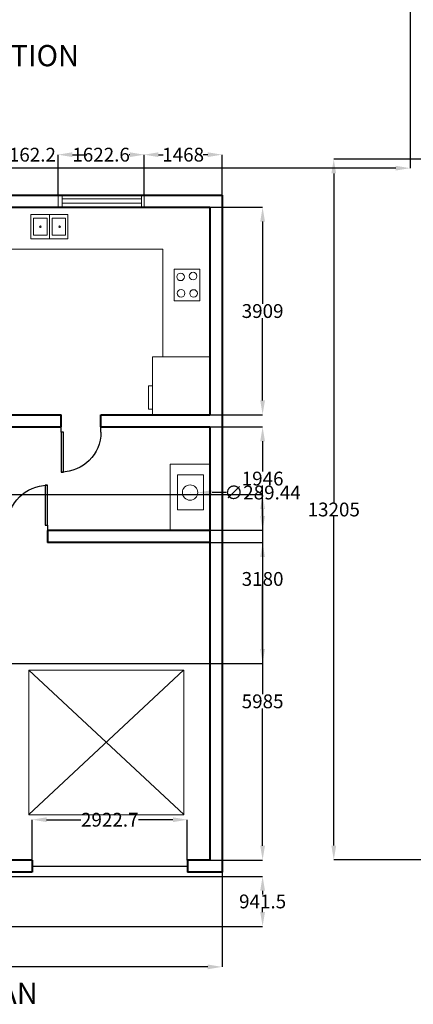
# Model space of a CAD drawing. Units: millimetres. Extents: x 23 to 3809233, y 4 to 290343.
# Tile 3 of 8: x 1908235 to 1915648, y 133276 to 151826. Entities that reach past the tile are written whole.
import ezdxf

# ---------------------------------------------------------------- set-up
doc = ezdxf.new("R2010")
doc.units = ezdxf.units.MM
doc.header["$MEASUREMENT"] = 0
for name, color, linetype, lineweight in [('A-ANNO-DIMS', 2, 'Continuous', 18), ('A-ANNO-TEXT', 7, 'Continuous', 25), ('A-DOOR', 3, 'Continuous', 25), ('A-EQPM', 8, 'Continuous', 18), ('A-FLOR-CASE', 8, 'Continuous', 20), ('A-FLOR-FIXT', 9, 'Continuous', 18), ('A-GLAZ', 4, 'Continuous', 18), ('A-WALL', 7, 'Continuous', 40)]:
    doc.layers.add(name, color=color, linetype=linetype, lineweight=lineweight)
doc.styles.get("Standard").update_dxf_attribs({"font": 'arial.ttf'})
doc.dimstyles.get("Standard").update_dxf_attribs({"dimtxt": 260.18, "dimasz": 270.18, "dimexe": 0.18, "dimexo": 0.0625, "dimgap": 0.09, "dimtad": 0, "dimtih": 1, "dimtoh": 1, "dimdec": 0, "dimzin": 0, "dimdsep": 46, "dimtxsty": 'Standard', "dimcen": 0.09, "dimadec": 0, "dimazin": 0, "dimtfac": 1, "dimtdec": 0, "dimtofl": 0, "dimtmove": 0, "dimatfit": 3, "dimfxl": 1, "dimtolj": 1, "dimtzin": 0, "dimarcsym": 0})

# ---------------------------------------------------------------- blocks, each defined once
blk = doc.blocks.new('*U2')
for p, q in [((0, 0), (0, -100)), ((750, 0), (750, -100))]:
    blk.add_line(p, q)
blk.add_lwpolyline([(0, 0), (0, 750), (43.75, 750), (43.75, 0)], close=True)
blk.add_arc((0, 0), 750, 0, 90)
blk = doc.blocks.new('*D48')
at = {"layer": 'A-ANNO-DIMS', "color": 0, "lineweight": -2, "transparency": 16777216}
for p, q in [((1898390, 135763), (1898390, 133980)), ((1912047, 135763), (1912047, 133980)), ((1898660, 133981), (1904741, 133981)), ((1911777, 133981), (1905696, 133981))]:
    blk.add_line(p, q, dxfattribs=at)
at = {"layer": 'A-ANNO-DIMS', "color": 0, "transparency": 16777216}
for points in [[(1898660, 134026), (1898660, 133936), (1898390, 133981)], [(1911777, 134026), (1911777, 133936), (1912047, 133981)]]:
    blk.add_solid(points, dxfattribs=at)
at = {"layer": 'Defpoints', "color": 0, "transparency": 16777216}
for p in [(1898390, 135763), (1912047, 135763), (1912047, 133981)]:
    blk.add_point(p, dxfattribs=at)
at = {"layer": 'A-ANNO-DIMS', "color": 0, "transparency": 16777216, "insert": (1905219, 133981), "char_height": 260.2, "attachment_point": 5}
blk.add_mtext('\\A1;13657', dxfattribs=at)
blk = doc.blocks.new('*D53')
at = {"layer": 'A-ANNO-DIMS', "color": 0, "lineweight": -2, "transparency": 16777216}
for p, q in [((1911819, 141976), (1912810, 141976)), ((1912810, 141706), (1912810, 139117)), ((1912810, 136262), (1912810, 138851)), ((1911819, 135992), (1912810, 135992))]:
    blk.add_line(p, q, dxfattribs=at)
at = {"layer": 'A-ANNO-DIMS', "color": 0, "transparency": 16777216}
for points in [[(1912765, 141706), (1912855, 141706), (1912810, 141976)], [(1912765, 136262), (1912855, 136262), (1912810, 135992)]]:
    blk.add_solid(points, dxfattribs=at)
at = {"layer": 'Defpoints', "color": 0, "transparency": 16777216}
for p in [(1911819, 141976), (1912810, 141976), (1911819, 135992)]:
    blk.add_point(p, dxfattribs=at)
at = {"layer": 'A-ANNO-DIMS', "color": 0, "transparency": 16777216, "insert": (1912810, 138984), "char_height": 260.2, "attachment_point": 5}
blk.add_mtext('\\A1;5985', dxfattribs=at)
blk = doc.blocks.new('*D54')
at = {"layer": 'A-ANNO-DIMS', "color": 0, "lineweight": -2, "transparency": 16777216}
for p, q in [((1911819, 144154), (1912810, 144154)), ((1912810, 143884), (1912810, 143314)), ((1912810, 142478), (1912810, 143048)), ((1911816, 142208), (1912810, 142208))]:
    blk.add_line(p, q, dxfattribs=at)
at = {"layer": 'A-ANNO-DIMS', "color": 0, "transparency": 16777216}
for points in [[(1912765, 143884), (1912855, 143884), (1912810, 144154)], [(1912765, 142478), (1912855, 142478), (1912810, 142208)]]:
    blk.add_solid(points, dxfattribs=at)
at = {"layer": 'Defpoints', "color": 0, "transparency": 16777216}
for p in [(1911819, 144154), (1912810, 144154), (1911816, 142208)]:
    blk.add_point(p, dxfattribs=at)
at = {"layer": 'A-ANNO-DIMS', "color": 0, "transparency": 16777216, "insert": (1912810, 143181), "char_height": 260.2, "attachment_point": 5}
blk.add_mtext('\\A1;1946', dxfattribs=at)
blk = doc.blocks.new('*D55')
at = {"layer": 'A-ANNO-DIMS', "color": 0, "lineweight": -2, "transparency": 16777216}
for p, q in [((1911819, 148292), (1912810, 148292)), ((1912810, 148022), (1912810, 146470)), ((1912810, 144653), (1912810, 146204)), ((1911816, 144382), (1912810, 144382))]:
    blk.add_line(p, q, dxfattribs=at)
at = {"layer": 'A-ANNO-DIMS', "color": 0, "transparency": 16777216}
for points in [[(1912765, 148022), (1912855, 148022), (1912810, 148292)], [(1912765, 144653), (1912855, 144653), (1912810, 144382)]]:
    blk.add_solid(points, dxfattribs=at)
at = {"layer": 'Defpoints', "color": 0, "transparency": 16777216}
for p in [(1911819, 148292), (1912810, 148292), (1911816, 144382)]:
    blk.add_point(p, dxfattribs=at)
at = {"layer": 'A-ANNO-DIMS', "color": 0, "transparency": 16777216, "insert": (1912810, 146337), "char_height": 260.2, "attachment_point": 5}
blk.add_mtext('\\A1;3909', dxfattribs=at)
blk = doc.blocks.new('*D64')
at = {"layer": 'A-ANNO-DIMS', "color": 0, "lineweight": -2, "transparency": 16777216}
for p, q in [((1907524.135363, 149282.788959), (1907253.955363, 149282.788959)), ((1907794.315363, 148291.751459), (1907794.315363, 149282.968959)), ((1908956.509231, 148520.351459), (1908956.509231, 149282.968959)), ((1909226.689231, 149282.788959), (1909496.869231, 149282.788959))]:
    blk.add_line(p, q, dxfattribs=at)
at = {"layer": 'A-ANNO-DIMS', "color": 0, "transparency": 16777216}
for points in [[(1907524.135363, 149327.818959), (1907524.135363, 149237.758959), (1907794.315363, 149282.788959)], [(1909226.689231, 149327.818959), (1909226.689231, 149237.758959), (1908956.509231, 149282.788959)]]:
    blk.add_solid(points, dxfattribs=at)
at = {"layer": 'Defpoints', "color": 0, "transparency": 16777216}
for p in [(1908956.509231, 149282.788959), (1908956.509231, 148520.288959), (1907794.315363, 148291.688959)]:
    blk.add_point(p, dxfattribs=at)
at = {"layer": 'A-ANNO-DIMS', "color": 0, "transparency": 16777216, "insert": (1908375.412297, 149282.788959), "char_height": 260.18, "attachment_point": 5}
blk.add_mtext('\\A1;1162.2', dxfattribs=at)
blk = doc.blocks.new('*D65')
at = {"layer": 'A-ANNO-DIMS', "color": 0, "lineweight": -2, "transparency": 16777216}
for p, q in [((1908957, 148520), (1908957, 149283)), ((1909227, 149283), (1909240, 149283)), ((1910309, 149283), (1910296, 149283)), ((1910579, 148520), (1910579, 149283))]:
    blk.add_line(p, q, dxfattribs=at)
at = {"layer": 'A-ANNO-DIMS', "color": 0, "transparency": 16777216}
for points in [[(1909227, 149328), (1909227, 149238), (1908957, 149283)], [(1910309, 149328), (1910309, 149238), (1910579, 149283)]]:
    blk.add_solid(points, dxfattribs=at)
at = {"layer": 'Defpoints', "color": 0, "transparency": 16777216}
for p in [(1910579, 149283), (1908957, 148520), (1910579, 148520)]:
    blk.add_point(p, dxfattribs=at)
at = {"layer": 'A-ANNO-DIMS', "color": 0, "transparency": 16777216, "insert": (1909768, 149283), "char_height": 260.2, "attachment_point": 5}
blk.add_mtext('\\A1;1622.6', dxfattribs=at)
blk = doc.blocks.new('*D66')
at = {"layer": 'A-ANNO-DIMS', "color": 0, "lineweight": -2, "transparency": 16777216}
for p, q in [((1910579, 148520), (1910579, 149283)), ((1910849, 149283), (1910937, 149283)), ((1911777, 149283), (1911690, 149283)), ((1912047, 148520), (1912047, 149283))]:
    blk.add_line(p, q, dxfattribs=at)
at = {"layer": 'A-ANNO-DIMS', "color": 0, "transparency": 16777216}
for points in [[(1910849, 149328), (1910849, 149238), (1910579, 149283)], [(1911777, 149328), (1911777, 149238), (1912047, 149283)]]:
    blk.add_solid(points, dxfattribs=at)
at = {"layer": 'Defpoints', "color": 0, "transparency": 16777216}
for p in [(1912047, 149283), (1910579, 148520), (1912047, 148520)]:
    blk.add_point(p, dxfattribs=at)
at = {"layer": 'A-ANNO-DIMS', "color": 0, "transparency": 16777216, "insert": (1911313, 149283), "char_height": 260.2, "attachment_point": 5}
blk.add_mtext('\\A1;1468', dxfattribs=at)
blk = doc.blocks.new('*D69')
at = {"layer": 'A-ANNO-DIMS', "color": 0, "lineweight": -2, "transparency": 16777216}
for p, q in [((1908470, 135992), (1908470, 136754)), ((1908740, 136754), (1909389, 136754)), ((1911122, 136754), (1910473, 136754)), ((1911392, 135992), (1911392, 136754))]:
    blk.add_line(p, q, dxfattribs=at)
at = {"layer": 'A-ANNO-DIMS', "color": 0, "transparency": 16777216}
for points in [[(1908740, 136799), (1908740, 136709), (1908470, 136754)], [(1911122, 136799), (1911122, 136709), (1911392, 136754)]]:
    blk.add_solid(points, dxfattribs=at)
at = {"layer": 'Defpoints', "color": 0, "transparency": 16777216}
for p in [(1911392, 136754), (1908470, 135992), (1911392, 135992)]:
    blk.add_point(p, dxfattribs=at)
at = {"layer": 'A-ANNO-DIMS', "color": 0, "transparency": 16777216, "insert": (1909931, 136754), "char_height": 260.2, "attachment_point": 5}
blk.add_mtext('\\A1;2922.7', dxfattribs=at)
blk = doc.blocks.new('*D71')
at = {"layer": 'A-ANNO-DIMS', "color": 0, "lineweight": -2, "transparency": 16777216}
for p, q in [((1905183, 142880), (1912810, 142880)), ((1912810, 142610), (1912810, 141423)), ((1912810, 139970), (1912810, 141157)), ((1905183, 139700), (1912810, 139700))]:
    blk.add_line(p, q, dxfattribs=at)
at = {"layer": 'A-ANNO-DIMS', "color": 0, "transparency": 16777216}
for points in [[(1912765, 142610), (1912855, 142610), (1912810, 142880)], [(1912765, 139970), (1912855, 139970), (1912810, 139700)]]:
    blk.add_solid(points, dxfattribs=at)
at = {"layer": 'Defpoints', "color": 0, "transparency": 16777216}
for p in [(1905183, 142880), (1912810, 142880), (1905183, 139700)]:
    blk.add_point(p, dxfattribs=at)
at = {"layer": 'A-ANNO-DIMS', "color": 0, "transparency": 16777216, "insert": (1912810, 141290), "char_height": 260.2, "attachment_point": 5}
blk.add_mtext('\\A1;3180', dxfattribs=at)
blk = doc.blocks.new('*D79')
at = {"layer": 'A-ANNO-DIMS', "color": 0, "lineweight": -2, "transparency": 16777216}
for p, q in [((1906678, 135685), (1912810, 135685)), ((1912810, 135414), (1912810, 135347)), ((1912810, 135013), (1912810, 135081)), ((1906678, 134743), (1912810, 134743))]:
    blk.add_line(p, q, dxfattribs=at)
at = {"layer": 'A-ANNO-DIMS', "color": 0, "transparency": 16777216}
for points in [[(1912765, 135414), (1912855, 135414), (1912810, 135685)], [(1912765, 135013), (1912855, 135013), (1912810, 134743)]]:
    blk.add_solid(points, dxfattribs=at)
at = {"layer": 'Defpoints', "color": 0, "transparency": 16777216}
for p in [(1906678, 135685), (1912810, 135685), (1906678, 134743)]:
    blk.add_point(p, dxfattribs=at)
at = {"layer": 'A-ANNO-DIMS', "color": 0, "transparency": 16777216, "insert": (1912810, 135214), "char_height": 260.2, "attachment_point": 5}
blk.add_mtext('\\A1;941.5', dxfattribs=at)
blk = doc.blocks.new('*D80')
at = {"layer": 'A-ANNO-DIMS', "color": 0, "lineweight": -2, "transparency": 16777216}
for p, q in [((1893468, 163690), (1893468, 149029)), ((1915588, 152264), (1915588, 149029)), ((1893739, 149029), (1904037, 149029)), ((1915318, 149029), (1905020, 149029))]:
    blk.add_line(p, q, dxfattribs=at)
at = {"layer": 'A-ANNO-DIMS', "color": 0, "transparency": 16777216}
for points in [[(1893739, 149074), (1893739, 148984), (1893468, 149029)], [(1915318, 149074), (1915318, 148984), (1915588, 149029)]]:
    blk.add_solid(points, dxfattribs=at)
at = {"layer": 'Defpoints', "color": 0, "transparency": 16777216}
for p in [(1893468, 163690), (1915588, 152265), (1915588, 149029)]:
    blk.add_point(p, dxfattribs=at)
at = {"layer": 'A-ANNO-DIMS', "color": 0, "transparency": 16777216, "insert": (1904528, 149029), "char_height": 260.2, "attachment_point": 5}
blk.add_mtext('\\A1;22120', dxfattribs=at)
blk = doc.blocks.new('*D117')
at = {"layer": 'A-ANNO-DIMS', "color": 0, "lineweight": -2, "transparency": 16777216}
for p, q in [((1929762, 149200), (1914150, 149200)), ((1914150, 148930), (1914150, 142731)), ((1914150, 136265), (1914150, 142465)), ((1918411, 135995), (1914150, 135995))]:
    blk.add_line(p, q, dxfattribs=at)
at = {"layer": 'A-ANNO-DIMS', "color": 0, "transparency": 16777216}
for points in [[(1914105, 148930), (1914195, 148930), (1914150, 149200)], [(1914105, 136265), (1914195, 136265), (1914150, 135995)]]:
    blk.add_solid(points, dxfattribs=at)
at = {"layer": 'Defpoints', "color": 0, "transparency": 16777216}
for p in [(1914150, 149200), (1929762, 149200), (1918411, 135995)]:
    blk.add_point(p, dxfattribs=at)
at = {"layer": 'A-ANNO-DIMS', "color": 0, "transparency": 16777216, "insert": (1914150, 142598), "char_height": 260.2, "attachment_point": 5}
blk.add_mtext('\\A1;13205', dxfattribs=at)
blk = doc.blocks.new('*D127')
at = {"layer": 'A-ANNO-DIMS', "color": 0, "lineweight": -2, "transparency": 16777216}
for p, q in [((1911443, 142918), (1911443, 142918)), ((1911443, 142918), (1911443, 142918)), ((1912128, 142918), (1911858, 142918))]:
    blk.add_line(p, q, dxfattribs=at)
at = {"layer": 'A-ANNO-DIMS', "color": 0, "transparency": 16777216}
blk.add_solid([(1911858, 142963), (1911858, 142873), (1911588, 142918)], dxfattribs=at)
at = {"layer": 'Defpoints', "color": 0, "transparency": 16777216}
for p in [(1911298, 142918), (1911588, 142918)]:
    blk.add_point(p, dxfattribs=at)
at = {"layer": 'A-ANNO-DIMS', "color": 0, "transparency": 16777216, "insert": (1912809, 142918), "char_height": 260.18, "attachment_point": 5}
blk.add_mtext('\\A1;∅289.44', dxfattribs=at)

msp = doc.modelspace()

# ---------------------------------------------------------------- linework, layer by layer
at = {"layer": 'A-DOOR'}
msp.add_line((1908469.731, 135877.389), (1911392.434, 135877.389), dxfattribs=at)
at = {"layer": 'A-EQPM'}
for p, q in [((1908409.259, 139573.019), (1911323.873, 136849.314)), ((1911320.873, 139573.019), (1908409.259, 136849.314))]:
    msp.add_line(p, q, dxfattribs=at)
for points in [[(1911143.931, 147120.08, -0.414213562), (1911146.931, 147123.08), (1911626.738, 147123.08, -0.414213562), (1911629.738, 147120.08), (1911629.738, 146530.897, -0.414213562), (1911626.738, 146527.897), (1911146.931, 146527.897, -0.414213562), (1911143.931, 146530.897)], [(1911818.654, 145472.116, 0.414213562), (1911815.654, 145475.116), (1910736.868, 145475.116, 0.414213562), (1910733.868, 145472.116), (1910733.868, 144385.478, 0.414213562), (1910736.868, 144382.478), (1911815.654, 144382.478, 0.414213562), (1911818.654, 144385.478)], [(1910733.868, 144925.797, 0.414213562), (1910730.868, 144928.797), (1910661.427, 144928.797, 0.414213562), (1910658.427, 144925.797), (1910658.427, 144492.893, 0.414213562), (1910661.427, 144489.893), (1910730.868, 144489.893, 0.414213562), (1910733.868, 144492.893)], [(1908406.259, 139570.019, -0.414213562), (1908409.259, 139573.019), (1911320.873, 139573.019, -0.414213562), (1911323.873, 139570.019), (1911323.873, 136849.314, -0.414213562), (1911320.873, 136846.314), (1908409.259, 136846.314, -0.414213562), (1908406.259, 136849.314)]]:
    msp.add_lwpolyline(points, format="xyb", close=True, dxfattribs=at)
for centre in [(1911265.852, 146981.031), (1911500.112, 146996.291), (1911273.49, 146670.764), (1911510.299, 146668.221)]:
    msp.add_circle(centre, 71.208, dxfattribs=at)
at = {"layer": 'A-FLOR-CASE'}
for p, q in [((1908018.892, 147503.249), (1910929.729, 147503.249)), ((1910929.729, 147503.249), (1910929.729, 145475.116)), ((1910929.729, 145475.116), (1911818.654, 145475.116))]:
    msp.add_line(p, q, dxfattribs=at)
at = {"layer": 'A-FLOR-FIXT'}
msp.add_line((1908793.459, 148156.716), (1908793.459, 147695.201), dxfattribs=at)
msp.add_lwpolyline([(1908443.683, 148156.716), (1909143.234, 148156.716), (1909143.234, 147695.201), (1908443.683, 147695.201)], close=True, dxfattribs=at)
for points in [[(1908495.983, 148083.153, -0.414213562), (1908498.983, 148086.153), (1908747.8, 148086.153, -0.414213562), (1908750.8, 148083.153), (1908750.8, 147766.619, -0.414213562), (1908747.8, 147763.619), (1908498.983, 147763.619, -0.414213562), (1908495.983, 147766.619)], [(1908843.67, 148083.153, -0.414213562), (1908846.67, 148086.153), (1909095.487, 148086.153, -0.414213562), (1909098.487, 148083.153), (1909098.487, 147766.619, -0.414213562), (1909095.487, 147763.619), (1908846.67, 147763.619, -0.414213562), (1908843.67, 147766.619)], [(1911818.654, 143448.998, 0.414213562), (1911815.654, 143451.998), (1911070.621, 143451.998, 0.414213562), (1911067.621, 143448.998), (1911067.621, 142207.876, 0.414213562), (1911070.621, 142204.876), (1911815.654, 142204.876, 0.414213562), (1911818.654, 142207.876)], [(1911694.266, 143247.447, 0.414213562), (1911691.266, 143250.447), (1911208.696, 143250.447, 0.414213562), (1911205.696, 143247.447), (1911205.696, 142595.754, 0.414213562), (1911208.696, 142592.754), (1911691.266, 142592.754, 0.414213562), (1911694.266, 142595.754)]]:
    msp.add_lwpolyline(points, format="xyb", close=True, dxfattribs=at)
for centre, radius in [((1908623.392, 147924.886), 15.119), ((1908986.197, 147924.886), 15.119), ((1911443.137, 142917.649), 144.721)]:
    msp.add_circle(centre, radius, dxfattribs=at)
at = {"layer": 'A-GLAZ'}
for p, q in [((1908956.509, 148520.289), (1908956.509, 148291.689)), ((1909037.053, 148520.289), (1909037.053, 148291.689)), ((1909037.053, 148450.918), (1910529.216, 148450.918)), ((1910529.216, 148520.289), (1910529.216, 148291.689)), ((1910579.153, 148520.289), (1910579.153, 148291.689)), ((1909037.053, 148368.638), (1910529.216, 148368.638))]:
    msp.add_line(p, q, dxfattribs=at)
at = {"layer": 'A-WALL'}
for p, q in [((1898390.054, 148520.289), (1912047.254, 148520.289)), ((1912047.254, 148520.289), (1912047.254, 135763.089)), ((1907794.315, 148291.689), (1911818.654, 148291.689)), ((1911818.654, 148291.689), (1911818.654, 144382.478)), ((1907794.315, 144382.478), (1909015.346, 144382.478)), ((1909015.346, 144153.878), (1909015.346, 144382.478)), ((1909765.346, 144153.878), (1909765.346, 144382.478)), ((1909765.346, 144382.478), (1910051.569, 144382.478)), ((1910051.569, 144382.478), (1911818.654, 144382.478)), ((1907794.315, 144153.878), (1909015.346, 144153.878)), ((1909765.346, 144153.878), (1910046.69, 144153.878)), ((1910046.69, 144153.878), (1911818.654, 144153.878)), ((1911818.654, 144153.878), (1911818.654, 135991.689)), ((1911818.654, 142577.621), (1911818.654, 135991.689)), ((1911818.654, 142204.876), (1908759.428, 142204.876)), ((1908759.428, 142204.876), (1908759.428, 141976.276)), ((1911818.654, 141976.276), (1908759.428, 141976.276)), ((1908469.731, 135991.689), (1907794.315, 135991.689)), ((1908469.731, 135991.689), (1908469.731, 135763.089)), ((1911818.654, 135991.689), (1911392.434, 135991.689)), ((1911392.434, 135991.689), (1911392.434, 135763.089)), ((1908469.731, 135763.089), (1907565.715, 135763.089)), ((1912047.254, 135763.089), (1911392.434, 135763.089))]:
    msp.add_line(p, q, dxfattribs=at)

# ---------------------------------------------------------------- block references
at = {"layer": 'A-DOOR', "xscale": -1, "rotation": 180}
msp.add_blockref('*U2', (1909015.346, 144053.878), dxfattribs=at)
at = {"layer": 'A-DOOR', "xscale": -1}
msp.add_blockref('*U2', (1908759.428, 142304.876), dxfattribs=at)

# ---------------------------------------------------------------- texts
at = {"layer": 'A-ANNO-TEXT', "char_height": 400, "attachment_point": 1}
for s, heights, insert in [('LEFT SIDE ELEVATION', [307.465], (1903808.34, 151348.696)), ('GROUND FLOOR PLAN', [0], (1902916.406, 133683.241))]:
    msp.add_mtext_dynamic_manual_height_columns(s, width=8410.77875, gutter_width=1, heights=heights, dxfattribs=dict(at, insert=insert))

# ---------------------------------------------------------------- dimensions: what is measured, and where the dimension line sits
at = {"layer": 'A-ANNO-DIMS'}
for base, p1, p2, override, picture, middle in [((1915588.32, 149029.101), (1893468.322, 163689.971), (1915588.32, 152264.531), {"dimdec": 0, "dimlfac": 1, "dimrnd": 0, "dimzin": 0, "dimdsep": 46, "dimlunit": 2}, '*D80', (1904528.321, 149029.101)), ((1908956.509, 149282.789), (1907794.315, 148291.689), (1908956.509, 148520.289), {"dimdec": 1, "dimlfac": 1, "dimrnd": 0, "dimzin": 0, "dimdsep": 46, "dimlunit": 2}, '*D64', (1908375.412, 149282.789)), ((1910579.153, 149282.789), (1908956.509, 148520.289), (1910579.153, 148520.289), {"dimdec": 1, "dimlfac": 1, "dimrnd": 0, "dimzin": 0, "dimdsep": 46, "dimlunit": 2}, '*D65', (1909767.831, 149282.789)), ((1912047.254, 149282.789), (1910579.153, 148520.289), (1912047.254, 148520.289), {"dimdec": 0, "dimlfac": 1, "dimrnd": 0, "dimzin": 0, "dimdsep": 46, "dimlunit": 2}, '*D66', (1911313.204, 149282.789)), ((1911392.434, 136754.189), (1908469.731, 135991.689), (1911392.434, 135991.689), {"dimdec": 1, "dimlfac": 1, "dimrnd": 0, "dimzin": 0, "dimdsep": 46, "dimlunit": 2}, '*D69', (1909931.082, 136754.189)), ((1912047.254, 133980.582), (1898390.054, 135763.089), (1912047.254, 135763.089), {"dimdec": 0, "dimlfac": 1, "dimrnd": 0, "dimzin": 0, "dimdsep": 46, "dimlunit": 2}, '*D48', (1905218.654, 133980.582))]:
    dim = msp.add_linear_dim(base=base, p1=p1, p2=p2, dimstyle='Standard', override=override, dxfattribs=at)
    dim.commit()
    dim.dimension.update_dxf_attribs({"geometry": picture, "text_midpoint": middle})
for base, p1, p2, override, picture, middle in [((1914149.758, 149200.29), (1918410.662, 135995.166), (1929762.389, 149200.29), {"dimdec": 0, "dimlfac": 1, "dimrnd": 0, "dimzin": 0, "dimdsep": 46, "dimlunit": 2}, '*D117', (1914149.758, 142597.728)), ((1912809.754, 148291.689), (1911815.654, 144382.478), (1911818.654, 148291.689), {"dimdec": 0, "dimlfac": 1, "dimrnd": 0, "dimzin": 0, "dimdsep": 46, "dimlunit": 2}, '*D55', (1912809.754, 146337.084)), ((1912809.754, 144153.878), (1911815.654, 142207.876), (1911818.654, 144153.878), {"dimdec": 0, "dimlfac": 1, "dimrnd": 0, "dimzin": 0, "dimdsep": 46, "dimlunit": 2}, '*D54', (1912809.754, 143180.877)), ((1912809.754, 142879.905), (1905183.132, 139699.662), (1905183.132, 142879.905), {"dimdec": 0, "dimlfac": 1, "dimrnd": 0, "dimzin": 0, "dimdsep": 46, "dimlunit": 2}, '*D71', (1912809.754, 141289.783)), ((1912809.754, 141976.276), (1911818.654, 135991.689), (1911818.654, 141976.276), {"dimdec": 0, "dimlfac": 1, "dimrnd": 0, "dimzin": 0, "dimdsep": 46, "dimlunit": 2}, '*D53', (1912809.754, 138983.982)), ((1912809.754, 135684.558), (1906677.88, 134743.082), (1906677.88, 135684.558), {"dimdec": 1, "dimlfac": 1, "dimrnd": 0, "dimzin": 0, "dimdsep": 46, "dimlunit": 2}, '*D79', (1912809.754, 135213.82))]:
    dim = msp.add_linear_dim(base=base, p1=p1, p2=p2, angle=90, dimstyle='Standard', override=override, dxfattribs=at)
    dim.commit()
    dim.dimension.update_dxf_attribs({"geometry": picture, "text_midpoint": middle})
dim = msp.add_diameter_dim_2p(p1=(1911298.416, 142917.65), p2=(1911587.859, 142917.649), dimstyle='Standard', override={"dimdec": 2, "dimlfac": 1, "dimrnd": 0, "dimzin": 0, "dimdsep": 46, "dimlunit": 2}, dxfattribs=at)
dim.commit()
dim.dimension.update_dxf_attribs({"geometry": '*D127', "text_midpoint": (1912128.219, 142917.648), "dimtype": 163})

doc.saveas('drawing.dxf')
